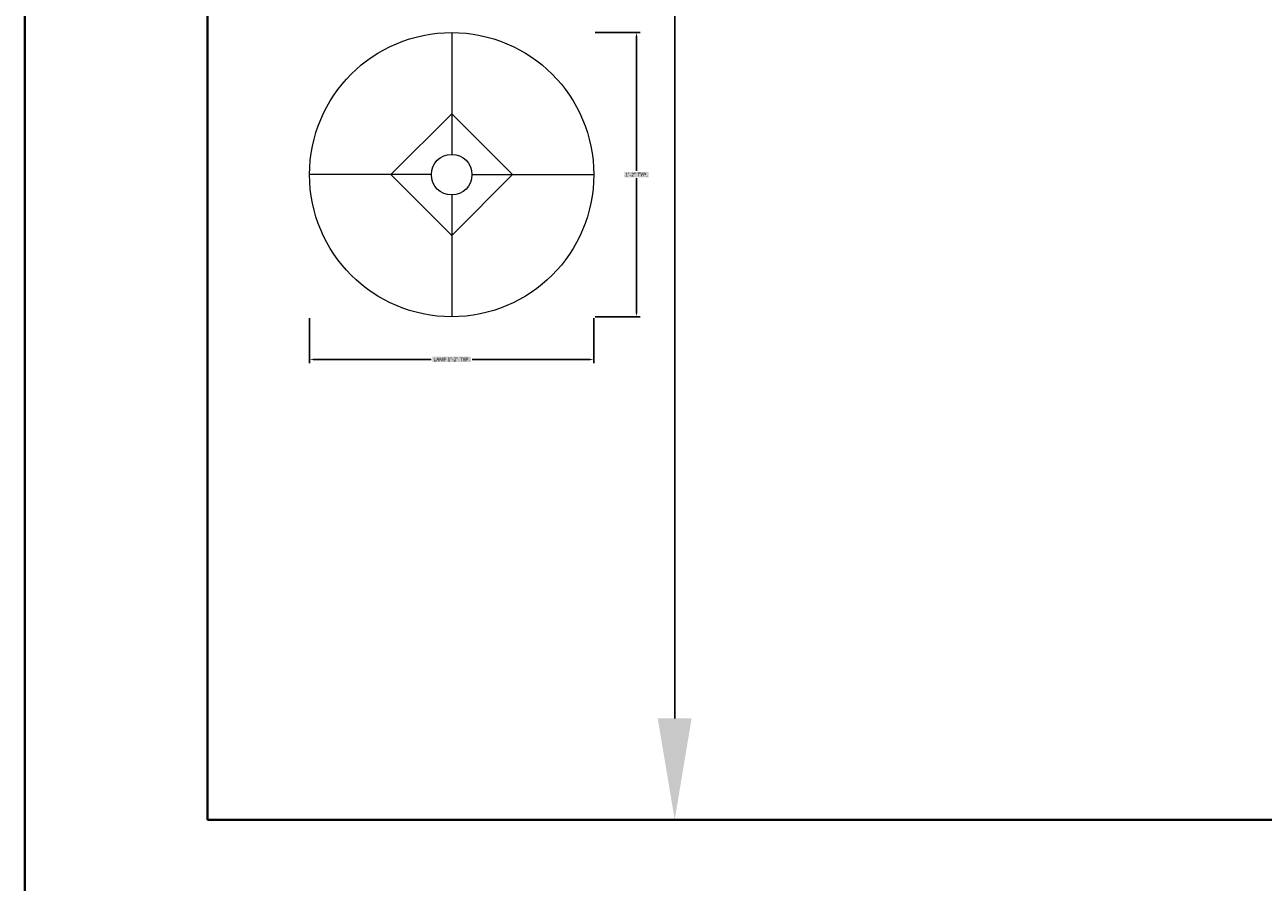
# Model space of a CAD drawing. Units: inches. Extents: x -301 to 715, y -607 to 364.
# Tile 57 of 141: x -205 to -144, y -218 to -176. Entities that reach past the tile are written whole.
import ezdxf

# ---------------------------------------------------------------- set-up
doc = ezdxf.new("R2010")
doc.units = ezdxf.units.IN
doc.header["$MEASUREMENT"] = 0
for name, color, linetype, lineweight in [('A-ANNO-DIMS', 2, 'Continuous', 18), ('A-FURN', 8, 'Continuous', 18), ('A-WALL', 3, 'Continuous', 40)]:
    doc.layers.add(name, color=color, linetype=linetype, lineweight=lineweight)
doc.styles.get("Standard").update_dxf_attribs({"font": 'arial.ttf'})
doc.dimstyles.get("Standard").update_dxf_attribs({"dimtxt": 0.18, "dimasz": 0.18, "dimexe": 0.18, "dimexo": 0.0625, "dimgap": 0.09, "dimtad": 0, "dimtih": 1, "dimtoh": 1, "dimdec": 1, "dimzin": 0, "dimdsep": 46, "dimlunit": 4, "dimtxsty": 'Standard', "dimcen": 0.09, "dimclrd": 3, "dimclre": 4, "dimclrt": 6, "dimadec": 0, "dimazin": 0, "dimtfac": 1, "dimtdec": 1, "dimtofl": 0, "dimtmove": 0, "dimatfit": 3, "dimfxl": 1, "dimtfill": 2, "dimtfillclr": 51, "dimtolj": 1, "dimtzin": 0, "dimarcsym": 0})

# ---------------------------------------------------------------- blocks, each defined once
blk = doc.blocks.new('Lamp - Table')
for p, q in [((0, 7), (0, 1)), ((0, 3), (-3, 0)), ((3, 0), (0, 3)), ((-1, 0), (-7, 0)), ((-3, 0), (0, -3)), ((0, -3), (3, 0)), ((1, 0), (7, 0)), ((0, -1), (0, -7))]:
    blk.add_line(p, q)
for radius in [7, 1]:
    blk.add_circle((0, 0), radius)
blk = doc.blocks.new('*D41')
at = {"layer": 'A-ANNO-DIMS', "color": 0, "lineweight": -2, "transparency": 16777216}
for p, q in [((-195.541, -73.318), (-172.412, -73.318)), ((-172.592, -78.318), (-172.592, -140.44)), ((-172.592, -209.818), (-172.592, -147.696)), ((-195.541, -214.818), (-172.412, -214.818))]:
    blk.add_line(p, q, dxfattribs=at)
at = {"layer": 'A-ANNO-DIMS', "color": 0, "transparency": 16777216}
for points in [[(-173.426, -78.318), (-171.759, -78.318), (-172.592, -73.318)], [(-173.426, -209.818), (-171.759, -209.818), (-172.592, -214.818)]]:
    blk.add_solid(points, dxfattribs=at)
at = {"layer": 'Defpoints', "color": 0, "transparency": 16777216}
for p in [(-195.603, -73.318), (-195.603, -214.818), (-172.592, -214.818)]:
    blk.add_point(p, dxfattribs=at)
at = {"layer": 'A-ANNO-DIMS', "color": 0, "transparency": 16777216, "insert": (-172.592, -144.068), "char_height": 3, "attachment_point": 5, "bg_fill": 1, "box_fill_scale": 1.25, "bg_fill_color": 51, "bg_fill_transparency": 0}
blk.add_mtext('\\A1;11\'-9{\\H1x;\\S1/2;}"', dxfattribs=at)
blk = doc.blocks.new('*D104')
at = {"layer": 'A-ANNO-DIMS', "color": 4, "lineweight": -2, "transparency": 16777216}
for p, q in [((-190.576, -190.098), (-190.576, -192.316)), ((-176.576, -190.098), (-176.576, -192.316))]:
    blk.add_line(p, q, dxfattribs=at)
at = {"layer": 'A-ANNO-DIMS', "color": 3, "lineweight": -2, "transparency": 16777216}
for p, q in [((-190.396, -192.136), (-184.588, -192.136)), ((-176.756, -192.136), (-182.564, -192.136))]:
    blk.add_line(p, q, dxfattribs=at)
at = {"layer": 'A-ANNO-DIMS', "color": 3, "transparency": 16777216}
for points in [[(-190.396, -192.106), (-190.396, -192.166), (-190.576, -192.136)], [(-176.756, -192.106), (-176.756, -192.166), (-176.576, -192.136)]]:
    blk.add_solid(points, dxfattribs=at)
at = {"layer": 'Defpoints', "color": 0, "transparency": 16777216}
for p in [(-190.576, -190.036), (-176.576, -190.036), (-176.576, -192.136)]:
    blk.add_point(p, dxfattribs=at)
at = {"layer": 'A-ANNO-DIMS', "color": 6, "transparency": 16777216, "insert": (-183.576, -192.136), "char_height": 0.18, "attachment_point": 5, "bg_fill": 1, "box_fill_scale": 1.25, "bg_fill_color": 51, "bg_fill_transparency": 0}
blk.add_mtext('\\A1;LAMP 1\'-2" TYP.', dxfattribs=at)
blk = doc.blocks.new('*D105')
at = {"layer": 'A-ANNO-DIMS', "color": 4, "lineweight": -2, "transparency": 16777216}
for p, q in [((-176.513, -176.036), (-174.296, -176.036)), ((-176.513, -190.036), (-174.296, -190.036))]:
    blk.add_line(p, q, dxfattribs=at)
at = {"layer": 'A-ANNO-DIMS', "color": 3, "lineweight": -2, "transparency": 16777216}
for p, q in [((-174.476, -176.216), (-174.476, -182.855)), ((-174.476, -189.856), (-174.476, -183.216))]:
    blk.add_line(p, q, dxfattribs=at)
at = {"layer": 'A-ANNO-DIMS', "color": 3, "transparency": 16777216}
for points in [[(-174.506, -176.216), (-174.446, -176.216), (-174.476, -176.036)], [(-174.506, -189.856), (-174.446, -189.856), (-174.476, -190.036)]]:
    blk.add_solid(points, dxfattribs=at)
at = {"layer": 'Defpoints', "color": 0, "transparency": 16777216}
for p in [(-176.576, -176.036), (-174.476, -176.036), (-176.576, -190.036)]:
    blk.add_point(p, dxfattribs=at)
at = {"layer": 'A-ANNO-DIMS', "color": 6, "transparency": 16777216, "insert": (-174.476, -183.036), "char_height": 0.18, "attachment_point": 5, "bg_fill": 1, "box_fill_scale": 1.25, "bg_fill_color": 51, "bg_fill_transparency": 0}
blk.add_mtext('\\A1;1\'-2" TYP.', dxfattribs=at)
blk = doc.blocks.new('*D151')
at = {"layer": 'A-ANNO-DIMS', "color": 4, "lineweight": -2, "transparency": 16777216}
for p, q in [((-204.603, -223.755), (-204.603, 359.612)), ((-45.603, -214.755), (-45.603, 359.612))]:
    blk.add_line(p, q, dxfattribs=at)
at = {"layer": 'A-ANNO-DIMS', "color": 3, "lineweight": -2, "transparency": 16777216}
for p, q in [((-204.423, 359.432), (-125.494, 359.432)), ((-45.783, 359.432), (-124.713, 359.432))]:
    blk.add_line(p, q, dxfattribs=at)
at = {"layer": 'A-ANNO-DIMS', "color": 3, "transparency": 16777216}
for points in [[(-204.423, 359.462), (-204.423, 359.402), (-204.603, 359.432)], [(-45.783, 359.462), (-45.783, 359.402), (-45.603, 359.432)]]:
    blk.add_solid(points, dxfattribs=at)
at = {"layer": 'Defpoints', "color": 0, "transparency": 16777216}
for p in [(-45.603, 359.432), (-45.603, -214.818), (-204.603, -223.818)]:
    blk.add_point(p, dxfattribs=at)
at = {"layer": 'A-ANNO-DIMS', "color": 6, "transparency": 16777216, "insert": (-125.103, 359.432), "char_height": 0.18, "attachment_point": 5, "bg_fill": 1, "box_fill_scale": 1.25, "bg_fill_color": 51, "bg_fill_transparency": 0}
blk.add_mtext('\\A1;13\'-3"', dxfattribs=at)

msp = doc.modelspace()

# ---------------------------------------------------------------- linework, layer by layer
at = {"layer": 'A-WALL'}
for p, q in [((-204.603, -67.318), (-204.603, -223.818)), ((-195.603, -73.318), (-195.603, -214.818)), ((-195.603, -214.818), (-45.603, -214.818))]:
    msp.add_line(p, q, dxfattribs=at)

# ---------------------------------------------------------------- block references
at = {"layer": 'A-FURN'}
msp.add_blockref('Lamp - Table', (-183.576, -183.036), dxfattribs=at)

# ---------------------------------------------------------------- dimensions: what is measured, and where the dimension line sits
at = {"layer": 'A-ANNO-DIMS'}
dim = msp.add_linear_dim(base=(-45.603, 359.432), p1=(-204.603, -223.818), p2=(-45.603, -214.818), dimstyle='Standard', override={"dimdec": 1, "dimlfac": 1, "dimrnd": 0, "dimzin": 1, "dimdsep": 46, "dimlunit": 4, "dimfrac": 2}, dxfattribs=at)
dim.commit()
dim.dimension.update_dxf_attribs({"geometry": '*D151', "text_midpoint": (-125.103, 359.432)})
dim = msp.add_linear_dim(base=(-172.592, -214.818), p1=(-195.603, -73.318), p2=(-195.603, -214.818), angle=90, dimstyle='Standard', override={"dimtxt": 3, "dimasz": 5, "dimclrd": 0, "dimclre": 0, "dimclrt": 0}, dxfattribs=at)
dim.commit()
dim.dimension.update_dxf_attribs({"geometry": '*D41', "text_midpoint": (-172.592, -144.068)})
dim = msp.add_linear_dim(base=(-174.476, -176.036), p1=(-176.576, -190.036), p2=(-176.576, -176.036), angle=90, text='<> TYP.', dimstyle='Standard', override={"dimdec": 1, "dimlfac": 1, "dimrnd": 0, "dimzin": 1, "dimdsep": 46, "dimlunit": 4, "dimfrac": 2}, dxfattribs=at)
dim.commit()
dim.dimension.update_dxf_attribs({"geometry": '*D105', "text_midpoint": (-174.476, -183.036)})
dim = msp.add_linear_dim(base=(-176.576, -192.136), p1=(-190.576, -190.036), p2=(-176.576, -190.036), text='LAMP <> TYP.', dimstyle='Standard', override={"dimdec": 1, "dimlfac": 1, "dimrnd": 0, "dimzin": 1, "dimdsep": 46, "dimlunit": 4, "dimfrac": 2}, dxfattribs=at)
dim.commit()
dim.dimension.update_dxf_attribs({"geometry": '*D104', "text_midpoint": (-183.576, -192.136)})

doc.saveas('drawing.dxf')
